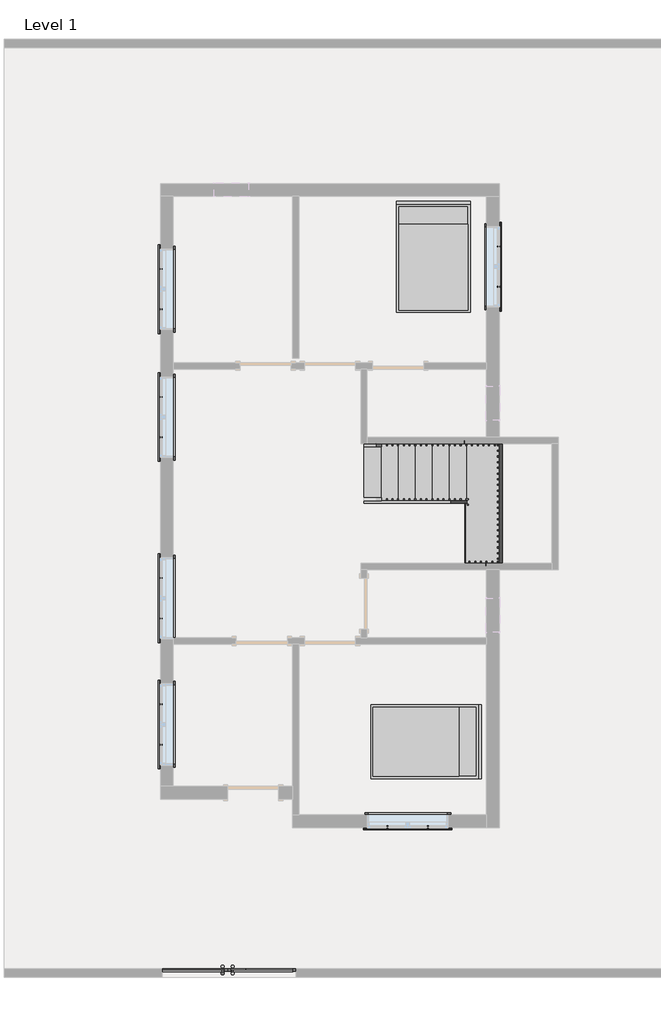
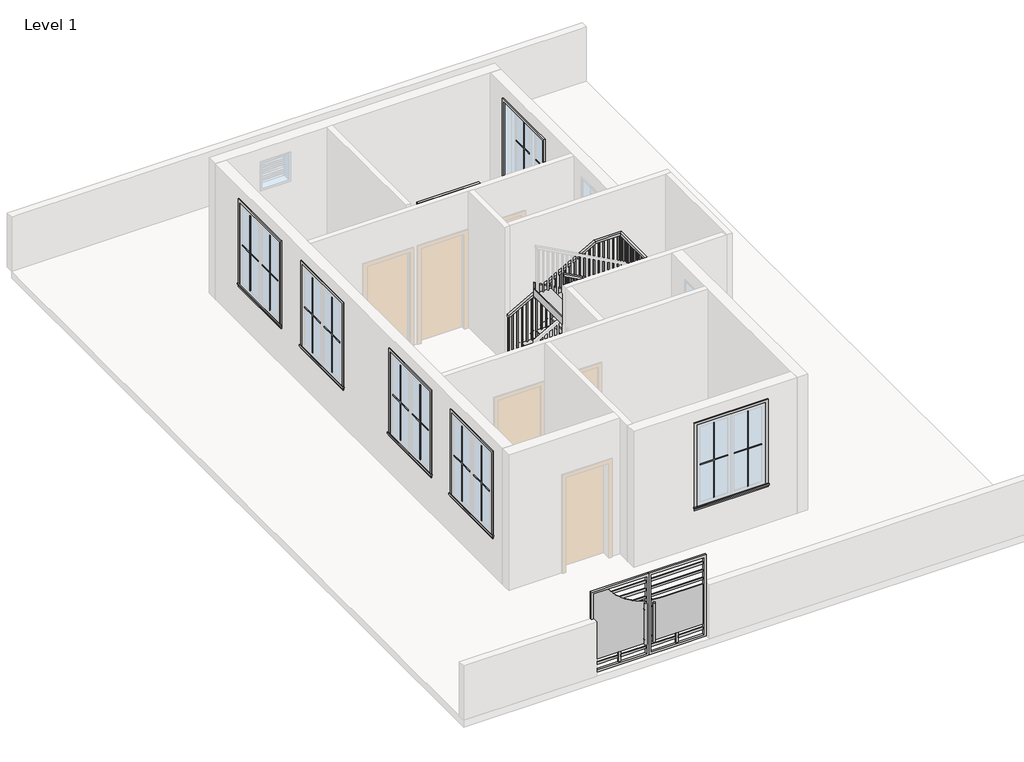
# One storey, part 2 of 2: 25 proxies, 5 members, 2 furniture elements, 1 railing, 1 stair flight.
"""IFC4 building model written with IfcOpenShell, lengths in millimetres."""

from ifc_helpers import new_model, si_unit, frame, origin, place, context, project, spatial, polyline, outline, extrude, faceted_brep, transform, mapped, element, save
from components import generic_models_113f6068, muntin_pattern_2x2_muntin_pattern_2x2_bff912c5, muntin_pattern_2x2_muntin_pattern_2x2_c2194282, trim_window_exterior_flat_with_sill_e04b3088, trim_window_interior_flat_picture_frame_2a7685fe, bed_17739_bed_17739_15c61121, stair_flight_5b4b54c9

model = new_model("IFC4")

# Units and contexts
model_context = context("Model", 3, world=origin())
ifc_project = project(units=[si_unit("LENGTHUNIT", "METRE", prefix="MILLI")], contexts=[model_context])

# Site, building, storey
site = spatial("IfcSite", under=ifc_project)
building = spatial("IfcBuilding", under=site)
storey = spatial("IfcBuildingStorey", under=building, Name="Level 1", Elevation=0.0)

# Proxies
placement = place(None, origin())
generic_models_shape = generic_models_113f6068(model_context)
element("IfcBuildingElementProxy", 1, Name="Generic Models", at=placement, inside=storey, context=model_context, shape_type="MappedRepresentation", body=[
    mapped(generic_models_shape, transform((-3606.0638307, -8534.8071204, 0.0), x_axis=(1.0, 0.0, 0.0), y_axis=(0.0, 1.0, 0.0), z_axis=(0.0, 0.0, 1.0))),
])
muntin_pattern_2x2_muntin_pattern_2x2_shape = muntin_pattern_2x2_muntin_pattern_2x2_bff912c5(model_context)
element("IfcBuildingElementProxy", 2, Name="Muntin Pattern_2x2 : Muntin Pattern_2x2", ObjectType="Muntin Pattern_2x2 : Muntin Pattern_2x2", at=placement, inside=storey, context=model_context, shape_type="MappedRepresentation", body=[
    mapped(muntin_pattern_2x2_muntin_pattern_2x2_shape, transform((-4796.6888307, -4528.6107799, 984.25), x_axis=(0.0, 1.0, 0.0), y_axis=(-1.0, 0.0, 0.0), z_axis=(0.0, 0.0, 1.0))),
])
element("IfcBuildingElementProxy", 3, Name="Muntin Pattern_2x2 : Muntin Pattern_2x2", ObjectType="Muntin Pattern_2x2 : Muntin Pattern_2x2", at=placement, inside=storey, context=model_context, shape_type="MappedRepresentation", body=[
    mapped(muntin_pattern_2x2_muntin_pattern_2x2_shape, transform((-4796.6888307, -2274.3607799, 984.25), x_axis=(0.0, 1.0, 0.0), y_axis=(-1.0, 0.0, 0.0), z_axis=(0.0, 0.0, 1.0))),
])
element("IfcBuildingElementProxy", 4, Name="Muntin Pattern_2x2 : Muntin Pattern_2x2", ObjectType="Muntin Pattern_2x2 : Muntin Pattern_2x2", at=placement, inside=storey, context=model_context, shape_type="MappedRepresentation", body=[
    mapped(muntin_pattern_2x2_muntin_pattern_2x2_shape, transform((-26.2513307, -6000.2232799, 984.25), x_axis=(-1.0, 0.0, 0.0), y_axis=(0.0, -1.0, 0.0), z_axis=(0.0, 0.0, 1.0))),
])
element("IfcBuildingElementProxy", 5, Name="Muntin Pattern_2x2 : Muntin Pattern_2x2", ObjectType="Muntin Pattern_2x2 : Muntin Pattern_2x2", at=placement, inside=storey, context=model_context, shape_type="MappedRepresentation", body=[
    mapped(muntin_pattern_2x2_muntin_pattern_2x2_shape, transform((1242.1611693, 4370.9142201, 984.25), x_axis=(0.0, -1.0, 0.0), y_axis=(1.0, 0.0, 0.0), z_axis=(0.0, 0.0, 1.0))),
])
element("IfcBuildingElementProxy", 6, Name="Muntin Pattern_2x2 : Muntin Pattern_2x2", ObjectType="Muntin Pattern_2x2 : Muntin Pattern_2x2", at=placement, inside=storey, context=model_context, shape_type="MappedRepresentation", body=[
    mapped(muntin_pattern_2x2_muntin_pattern_2x2_shape, transform((-4796.6888307, 3250.1392201, 984.25), x_axis=(0.0, 1.0, 0.0), y_axis=(-1.0, 0.0, 0.0), z_axis=(0.0, 0.0, 1.0))),
])
element("IfcBuildingElementProxy", 7, Name="Muntin Pattern_2x2 : Muntin Pattern_2x2", ObjectType="Muntin Pattern_2x2 : Muntin Pattern_2x2", at=placement, inside=storey, context=model_context, shape_type="MappedRepresentation", body=[
    mapped(muntin_pattern_2x2_muntin_pattern_2x2_shape, transform((-4796.6888307, 964.1392201, 984.25), x_axis=(0.0, 1.0, 0.0), y_axis=(-1.0, 0.0, 0.0), z_axis=(0.0, 0.0, 1.0))),
])
muntin_pattern_2x2_muntin_pattern_2x2_2_shape = muntin_pattern_2x2_muntin_pattern_2x2_c2194282(model_context)
element("IfcBuildingElementProxy", 8, Name="Muntin Pattern_2x2 : Muntin Pattern_2x2", ObjectType="Muntin Pattern_2x2 : Muntin Pattern_2x2", at=placement, inside=storey, context=model_context, shape_type="MappedRepresentation", body=[
    mapped(muntin_pattern_2x2_muntin_pattern_2x2_2_shape, transform((-4796.6888307, -3807.8857799, 984.25), x_axis=(0.0, -1.0, 0.0), y_axis=(1.0, 0.0, 0.0), z_axis=(0.0, 0.0, 1.0))),
])
element("IfcBuildingElementProxy", 9, Name="Muntin Pattern_2x2 : Muntin Pattern_2x2", ObjectType="Muntin Pattern_2x2 : Muntin Pattern_2x2", at=placement, inside=storey, context=model_context, shape_type="MappedRepresentation", body=[
    mapped(muntin_pattern_2x2_muntin_pattern_2x2_2_shape, transform((-4796.6888307, -1553.6357799, 984.25), x_axis=(0.0, -1.0, 0.0), y_axis=(1.0, 0.0, 0.0), z_axis=(0.0, 0.0, 1.0))),
])
element("IfcBuildingElementProxy", 10, Name="Muntin Pattern_2x2 : Muntin Pattern_2x2", ObjectType="Muntin Pattern_2x2 : Muntin Pattern_2x2", at=placement, inside=storey, context=model_context, shape_type="MappedRepresentation", body=[
    mapped(muntin_pattern_2x2_muntin_pattern_2x2_2_shape, transform((-746.9763307, -6000.2232799, 984.25), x_axis=(1.0, 0.0, 0.0), y_axis=(0.0, 1.0, 0.0), z_axis=(0.0, 0.0, 1.0))),
])
element("IfcBuildingElementProxy", 11, Name="Muntin Pattern_2x2 : Muntin Pattern_2x2", ObjectType="Muntin Pattern_2x2 : Muntin Pattern_2x2", at=placement, inside=storey, context=model_context, shape_type="MappedRepresentation", body=[
    mapped(muntin_pattern_2x2_muntin_pattern_2x2_2_shape, transform((1242.1611693, 3650.1892201, 984.25), x_axis=(0.0, 1.0, 0.0), y_axis=(-1.0, 0.0, 0.0), z_axis=(0.0, 0.0, 1.0))),
])
element("IfcBuildingElementProxy", 12, Name="Muntin Pattern_2x2 : Muntin Pattern_2x2", ObjectType="Muntin Pattern_2x2 : Muntin Pattern_2x2", at=placement, inside=storey, context=model_context, shape_type="MappedRepresentation", body=[
    mapped(muntin_pattern_2x2_muntin_pattern_2x2_2_shape, transform((-4796.6888307, 3970.8642201, 984.25), x_axis=(0.0, -1.0, 0.0), y_axis=(1.0, 0.0, 0.0), z_axis=(0.0, 0.0, 1.0))),
])
element("IfcBuildingElementProxy", 13, Name="Muntin Pattern_2x2 : Muntin Pattern_2x2", ObjectType="Muntin Pattern_2x2 : Muntin Pattern_2x2", at=placement, inside=storey, context=model_context, shape_type="MappedRepresentation", body=[
    mapped(muntin_pattern_2x2_muntin_pattern_2x2_2_shape, transform((-4796.6888307, 1684.8642201, 984.25), x_axis=(0.0, -1.0, 0.0), y_axis=(1.0, 0.0, 0.0), z_axis=(0.0, 0.0, 1.0))),
])
trim_window_exterior_flat_with_sill_shape = trim_window_exterior_flat_with_sill_e04b3088(model_context)
element("IfcBuildingElementProxy", 14, Name="Trim-Window-Exterior-Flat : with Sill", ObjectType="Trim-Window-Exterior-Flat : with Sill", at=placement, inside=storey, context=model_context, shape_type="MappedRepresentation", body=[
    mapped(trim_window_exterior_flat_with_sill_shape, transform((-4806.2138307, -4168.2482799, 2743.2), x_axis=(0.0, -1.0, 0.0), y_axis=(0.0, 0.0, 1.0), z_axis=(-1.0, 0.0, 0.0))),
])
element("IfcBuildingElementProxy", 15, Name="Trim-Window-Exterior-Flat : with Sill", ObjectType="Trim-Window-Exterior-Flat : with Sill", at=placement, inside=storey, context=model_context, shape_type="MappedRepresentation", body=[
    mapped(trim_window_exterior_flat_with_sill_shape, transform((-4806.2138307, -1913.9982799, 2743.2), x_axis=(0.0, -1.0, 0.0), y_axis=(0.0, 0.0, 1.0), z_axis=(-1.0, 0.0, 0.0))),
])
element("IfcBuildingElementProxy", 16, Name="Trim-Window-Exterior-Flat : with Sill", ObjectType="Trim-Window-Exterior-Flat : with Sill", at=placement, inside=storey, context=model_context, shape_type="MappedRepresentation", body=[
    mapped(trim_window_exterior_flat_with_sill_shape, transform((-386.6138307, -6009.7482799, 2743.2), x_axis=(1.0, 0.0, 0.0), y_axis=(0.0, 0.0, 1.0), z_axis=(0.0, -1.0, 0.0))),
])
element("IfcBuildingElementProxy", 17, Name="Trim-Window-Exterior-Flat : with Sill", ObjectType="Trim-Window-Exterior-Flat : with Sill", at=placement, inside=storey, context=model_context, shape_type="MappedRepresentation", body=[
    mapped(trim_window_exterior_flat_with_sill_shape, transform((1251.6861693, 4010.5517201, 2743.2), x_axis=(0.0, 1.0, 0.0), y_axis=(0.0, 0.0, 1.0), z_axis=(1.0, 0.0, 0.0))),
])
element("IfcBuildingElementProxy", 18, Name="Trim-Window-Exterior-Flat : with Sill", ObjectType="Trim-Window-Exterior-Flat : with Sill", at=placement, inside=storey, context=model_context, shape_type="MappedRepresentation", body=[
    mapped(trim_window_exterior_flat_with_sill_shape, transform((-4806.2138307, 3610.5017201, 2743.2), x_axis=(0.0, -1.0, 0.0), y_axis=(0.0, 0.0, 1.0), z_axis=(-1.0, 0.0, 0.0))),
])
element("IfcBuildingElementProxy", 19, Name="Trim-Window-Exterior-Flat : with Sill", ObjectType="Trim-Window-Exterior-Flat : with Sill", at=placement, inside=storey, context=model_context, shape_type="MappedRepresentation", body=[
    mapped(trim_window_exterior_flat_with_sill_shape, transform((-4806.2138307, 1324.5017201, 2743.2), x_axis=(0.0, -1.0, 0.0), y_axis=(0.0, 0.0, 1.0), z_axis=(-1.0, 0.0, 0.0))),
])
trim_window_interior_flat_picture_frame_shape = trim_window_interior_flat_picture_frame_2a7685fe(model_context)
element("IfcBuildingElementProxy", 20, Name="Trim-Window-Interior-Flat : Picture Frame", ObjectType="Trim-Window-Interior-Flat : Picture Frame", at=placement, inside=storey, context=model_context, shape_type="MappedRepresentation", body=[
    mapped(trim_window_interior_flat_picture_frame_shape, transform((-4577.6138307, -4168.2482799, 2743.2), x_axis=(0.0, 1.0, 0.0), y_axis=(0.0, 0.0, 1.0), z_axis=(1.0, 0.0, 0.0))),
])
element("IfcBuildingElementProxy", 21, Name="Trim-Window-Interior-Flat : Picture Frame", ObjectType="Trim-Window-Interior-Flat : Picture Frame", at=placement, inside=storey, context=model_context, shape_type="MappedRepresentation", body=[
    mapped(trim_window_interior_flat_picture_frame_shape, transform((-4577.6138307, -1913.9982799, 2743.2), x_axis=(0.0, 1.0, 0.0), y_axis=(0.0, 0.0, 1.0), z_axis=(1.0, 0.0, 0.0))),
])
element("IfcBuildingElementProxy", 22, Name="Trim-Window-Interior-Flat : Picture Frame", ObjectType="Trim-Window-Interior-Flat : Picture Frame", at=placement, inside=storey, context=model_context, shape_type="MappedRepresentation", body=[
    mapped(trim_window_interior_flat_picture_frame_shape, transform((-386.6138307, -5781.1482799, 2743.2), x_axis=(-1.0, 0.0, 0.0), y_axis=(0.0, 0.0, 1.0), z_axis=(0.0, 1.0, 0.0))),
])
element("IfcBuildingElementProxy", 23, Name="Trim-Window-Interior-Flat : Picture Frame", ObjectType="Trim-Window-Interior-Flat : Picture Frame", at=placement, inside=storey, context=model_context, shape_type="MappedRepresentation", body=[
    mapped(trim_window_interior_flat_picture_frame_shape, transform((1023.0861693, 4010.5517201, 2743.2), x_axis=(0.0, -1.0, 0.0), y_axis=(0.0, 0.0, 1.0), z_axis=(-1.0, 0.0, 0.0))),
])
element("IfcBuildingElementProxy", 24, Name="Trim-Window-Interior-Flat : Picture Frame", ObjectType="Trim-Window-Interior-Flat : Picture Frame", at=placement, inside=storey, context=model_context, shape_type="MappedRepresentation", body=[
    mapped(trim_window_interior_flat_picture_frame_shape, transform((-4577.6138307, 3610.5017201, 2743.2), x_axis=(0.0, 1.0, 0.0), y_axis=(0.0, 0.0, 1.0), z_axis=(1.0, 0.0, 0.0))),
])
element("IfcBuildingElementProxy", 25, Name="Trim-Window-Interior-Flat : Picture Frame", ObjectType="Trim-Window-Interior-Flat : Picture Frame", at=placement, inside=storey, context=model_context, shape_type="MappedRepresentation", body=[
    mapped(trim_window_interior_flat_picture_frame_shape, transform((-4577.6138307, 1324.5017201, 2743.2), x_axis=(0.0, 1.0, 0.0), y_axis=(0.0, 0.0, 1.0), z_axis=(1.0, 0.0, 0.0))),
])

# Furniture
bed_17739_bed_17739_shape = bed_17739_bed_17739_15c61121(model_context)
element("IfcFurniture", 26, ObjectType="Bed_17739 : Bed_17739", at=placement, inside=storey, context=model_context, shape_type="MappedRepresentation", body=[
    mapped(bed_17739_bed_17739_shape, transform((70.5861693, 4162.9517201, 0.0), x_axis=(1.0, 0.0, 0.0), y_axis=(0.0, 1.0, 0.0), z_axis=(0.0, 0.0, 1.0))),
])
element("IfcFurniture", 27, ObjectType="Bed_17739 : Bed_17739", at=placement, inside=storey, context=model_context, shape_type="MappedRepresentation", body=[
    mapped(bed_17739_bed_17739_shape, transform((-81.8138307, -4473.0482799, 0.0), x_axis=(0.0, -1.0, 0.0), y_axis=(1.0, 0.0, 0.0), z_axis=(0.0, 0.0, 1.0))),
])

# Members
element("IfcMember", 28, ObjectType="Stringer - 2\" Width", at=placement, inside=storey, context=model_context, shape_type="SweptSolid", body=[
    extrude(outline(polyline([(204.070617, -1167.6638307), (0.0, -1167.6638307), (0.0, -907.3693279), (1199.4752762, 1251.6861693), (1261.5333333, 1251.6861693), (1261.5333333, 735.7690587), (204.070617, -1167.6638307)])), frame((0.0, 848.2517201, 0.0), z_axis=(0.0, 1.0, 0.0), x_axis=(0.0, 0.0, 1.0)), (0.0, 0.0, 1.0), 50.8),
])
element("IfcMember", 29, ObjectType="Stringer - 2\" Width", at=placement, inside=storey, context=model_context, shape_type="SweptSolid", body=[
    extrude(outline(polyline([(1251.6861693, 899.0517201), (1302.4861693, 899.0517201), (1302.4861693, -1285.3482799), (1251.6861693, -1285.3482799), (1251.6861693, 899.0517201)])), frame((0.0, 0.0, 956.7333333), z_axis=(0.0, 0.0, 1.0), x_axis=(1.0, 0.0, 0.0)), (0.0, 0.0, 1.0), 304.8),
])
element("IfcMember", 30, ObjectType="Stringer - 2\" Width", at=placement, inside=storey, context=model_context, shape_type="SweptSolid", body=[
    extrude(outline(polyline([(956.7333333, 1302.4861693), (1040.1539503, 1302.4861693), (2423.0428392, -1186.7138307), (2074.3641651, -1186.7138307), (956.7333333, 825.0216665), (956.7333333, 1302.4861693)])), frame((0.0, -1336.1482799, 0.0), z_axis=(0.0, 1.0, 0.0), x_axis=(0.0, 0.0, 1.0)), (0.0, 0.0, 1.0), 50.8),
])
element("IfcMember", 31, ObjectType="Stringer - 2\" Width", at=placement, inside=storey, context=model_context, shape_type="SweptSolid", body=[
    extrude(outline(polyline([(204.070617, -1167.6638307), (0.0, -1167.6638307), (0.0, -907.3693279), (846.6974984, 616.6861693), (1195.3761726, 616.6861693), (204.070617, -1167.6638307)])), frame((0.0, -218.5482799, 0.0), z_axis=(0.0, 1.0, 0.0), x_axis=(0.0, 0.0, 1.0)), (0.0, 0.0, 1.0), 50.8),
])
element("IfcMember", 32, ObjectType="Stringer - 2\" Width", at=placement, inside=storey, context=model_context, shape_type="SweptSolid", body=[
    extrude(outline(polyline([(1044.253054, 667.4861693), (1392.9317281, 667.4861693), (2423.0428392, -1186.7138307), (2074.3641651, -1186.7138307), (1044.253054, 667.4861693)])), frame((0.0, -218.5482799, 0.0), z_axis=(0.0, 1.0, 0.0), x_axis=(0.0, 0.0, 1.0)), (0.0, 0.0, 1.0), 50.8),
])

# Railing
element("IfcRailing", 33, ObjectType="Handrail - Rectangular", at=placement, inside=storey, context=model_context, shape_type="SolidModel", body=[
    faceted_brep([(-1167.6638307, 848.2517201, 1083.7333333), (-1167.6638307, 848.2517201, 1025.6675836), (-1167.6638307, 797.4517201, 1025.6675836), (-1167.6638307, 797.4517201, 1083.7333333), (667.4861693, 848.2517201, 2099.7333333), (680.6099298, 848.2517201, 2048.9333333), (680.6099298, 797.4517201, 2048.9333333), (667.4861693, 797.4517201, 2099.7333333), (1251.6861693, 848.2517201, 2099.7333333), (1251.6861693, 848.2517201, 2048.9333333), (1200.8861693, 797.4517201, 2048.9333333), (1200.8861693, 797.4517201, 2099.7333333), (1251.6861693, -1285.3482799, 2099.7333333), (1251.6861693, -1285.3482799, 2048.9333333), (1200.8861693, -1234.5482799, 2048.9333333), (1200.8861693, -1234.5482799, 2099.7333333), (976.5195026, -1285.3482799, 2099.7333333), (963.5139215, -1285.3482799, 2048.9333333), (963.5139215, -1234.5482799, 2048.9333333), (976.5195026, -1234.5482799, 2099.7333333), (-1186.7138307, -1285.3482799, 3285.0666667), (-1186.7138307, -1234.5482799, 3285.0666667), (-1186.7138307, -1234.5482799, 3227.1403208), (-1186.7138307, -1285.3482799, 3227.1403208)], [[[0, 1, 2, 3]], [[1, 0, 4, 5]], [[2, 1, 5, 6]], [[3, 2, 6, 7]], [[0, 3, 7, 4]], [[5, 4, 8, 9]], [[6, 5, 9, 10]], [[7, 6, 10, 11]], [[4, 7, 11, 8]], [[9, 8, 12, 13]], [[10, 9, 13, 14]], [[11, 10, 14, 15]], [[8, 11, 15, 12]], [[13, 12, 16, 17]], [[14, 13, 17, 18]], [[15, 14, 18, 19]], [[12, 15, 19, 16]], [[20, 21, 22, 23]], [[17, 16, 20, 23]], [[18, 17, 23, 22]], [[19, 18, 22, 21]], [[16, 19, 21, 20]]]),
    extrude(outline(polyline([(3190.6060742, -1120.0388307), (2201.3333333, -1120.0388307), (2201.3333333, -1100.9888307), (3180.1677181, -1100.9888307), (3190.6060742, -1120.0388307)])), frame((0.0, -1269.4732799, 0.0), z_axis=(0.0, 1.0, 0.0), x_axis=(0.0, 0.0, 1.0)), (0.0, 0.0, 1.0), 19.05),
    extrude(outline(polyline([(3134.9348414, -1018.4388307), (2201.3333333, -1018.4388307), (2201.3333333, -999.3888307), (3124.4964852, -999.3888307), (3134.9348414, -1018.4388307)])), frame((0.0, -1269.4732799, 0.0), z_axis=(0.0, 1.0, 0.0), x_axis=(0.0, 0.0, 1.0)), (0.0, 0.0, 1.0), 19.05),
    extrude(outline(polyline([(3079.2636085, -916.8388307), (2201.3333333, -916.8388307), (2201.3333333, -897.7888307), (3068.8252523, -897.7888307), (3079.2636085, -916.8388307)])), frame((0.0, -1269.4732799, 0.0), z_axis=(0.0, 1.0, 0.0), x_axis=(0.0, 0.0, 1.0)), (0.0, 0.0, 1.0), 19.05),
    extrude(outline(polyline([(3023.5923756, -815.2388307), (2032.0, -815.2388307), (2032.0, -796.1888307), (3013.1540195, -796.1888307), (3023.5923756, -815.2388307)])), frame((0.0, -1269.4732799, 0.0), z_axis=(0.0, 1.0, 0.0), x_axis=(0.0, 0.0, 1.0)), (0.0, 0.0, 1.0), 19.05),
    extrude(outline(polyline([(2967.9211427, -713.6388307), (2032.0, -713.6388307), (2032.0, -694.5888307), (2957.4827866, -694.5888307), (2967.9211427, -713.6388307)])), frame((0.0, -1269.4732799, 0.0), z_axis=(0.0, 1.0, 0.0), x_axis=(0.0, 0.0, 1.0)), (0.0, 0.0, 1.0), 19.05),
    extrude(outline(polyline([(2912.2499099, -612.0388307), (2032.0, -612.0388307), (2032.0, -592.9888307), (2901.8115537, -592.9888307), (2912.2499099, -612.0388307)])), frame((0.0, -1269.4732799, 0.0), z_axis=(0.0, 1.0, 0.0), x_axis=(0.0, 0.0, 1.0)), (0.0, 0.0, 1.0), 19.05),
    extrude(outline(polyline([(2856.578677, -510.4388307), (1862.6666667, -510.4388307), (1862.6666667, -491.3888307), (2846.1403208, -491.3888307), (2856.578677, -510.4388307)])), frame((0.0, -1269.4732799, 0.0), z_axis=(0.0, 1.0, 0.0), x_axis=(0.0, 0.0, 1.0)), (0.0, 0.0, 1.0), 19.05),
    extrude(outline(polyline([(2800.9074441, -408.8388307), (1862.6666667, -408.8388307), (1862.6666667, -389.7888307), (2790.4690879, -389.7888307), (2800.9074441, -408.8388307)])), frame((0.0, -1269.4732799, 0.0), z_axis=(0.0, 1.0, 0.0), x_axis=(0.0, 0.0, 1.0)), (0.0, 0.0, 1.0), 19.05),
    extrude(outline(polyline([(2745.2362112, -307.2388307), (1862.6666667, -307.2388307), (1862.6666667, -288.1888307), (2734.7978551, -288.1888307), (2745.2362112, -307.2388307)])), frame((0.0, -1269.4732799, 0.0), z_axis=(0.0, 1.0, 0.0), x_axis=(0.0, 0.0, 1.0)), (0.0, 0.0, 1.0), 19.05),
    extrude(outline(polyline([(2689.5649784, -205.6388307), (1693.3333333, -205.6388307), (1693.3333333, -186.5888307), (2679.1266222, -186.5888307), (2689.5649784, -205.6388307)])), frame((0.0, -1269.4732799, 0.0), z_axis=(0.0, 1.0, 0.0), x_axis=(0.0, 0.0, 1.0)), (0.0, 0.0, 1.0), 19.05),
    extrude(outline(polyline([(2633.8937455, -104.0388307), (1693.3333333, -104.0388307), (1693.3333333, -84.9888307), (2623.4553893, -84.9888307), (2633.8937455, -104.0388307)])), frame((0.0, -1269.4732799, 0.0), z_axis=(0.0, 1.0, 0.0), x_axis=(0.0, 0.0, 1.0)), (0.0, 0.0, 1.0), 19.05),
    extrude(outline(polyline([(2578.2225126, -2.4388307), (1693.3333333, -2.4388307), (1693.3333333, 16.6111693), (2567.7841564, 16.6111693), (2578.2225126, -2.4388307)])), frame((0.0, -1269.4732799, 0.0), z_axis=(0.0, 1.0, 0.0), x_axis=(0.0, 0.0, 1.0)), (0.0, 0.0, 1.0), 19.05),
    extrude(outline(polyline([(2522.5512797, 99.1611693), (1524.0, 99.1611693), (1524.0, 118.2111693), (2512.1129236, 118.2111693), (2522.5512797, 99.1611693)])), frame((0.0, -1269.4732799, 0.0), z_axis=(0.0, 1.0, 0.0), x_axis=(0.0, 0.0, 1.0)), (0.0, 0.0, 1.0), 19.05),
    extrude(outline(polyline([(2466.8800469, 200.7611693), (1524.0, 200.7611693), (1524.0, 219.8111693), (2456.4416907, 219.8111693), (2466.8800469, 200.7611693)])), frame((0.0, -1269.4732799, 0.0), z_axis=(0.0, 1.0, 0.0), x_axis=(0.0, 0.0, 1.0)), (0.0, 0.0, 1.0), 19.05),
    extrude(outline(polyline([(2411.208814, 302.3611693), (1524.0, 302.3611693), (1524.0, 321.4111693), (2400.7704578, 321.4111693), (2411.208814, 302.3611693)])), frame((0.0, -1269.4732799, 0.0), z_axis=(0.0, 1.0, 0.0), x_axis=(0.0, 0.0, 1.0)), (0.0, 0.0, 1.0), 19.05),
    extrude(outline(polyline([(2355.5375811, 403.9611693), (1354.6666667, 403.9611693), (1354.6666667, 423.0111693), (2345.0992249, 423.0111693), (2355.5375811, 403.9611693)])), frame((0.0, -1269.4732799, 0.0), z_axis=(0.0, 1.0, 0.0), x_axis=(0.0, 0.0, 1.0)), (0.0, 0.0, 1.0), 19.05),
    extrude(outline(polyline([(2299.8663482, 505.5611693), (1354.6666667, 505.5611693), (1354.6666667, 524.6111693), (2289.4279921, 524.6111693), (2299.8663482, 505.5611693)])), frame((0.0, -1269.4732799, 0.0), z_axis=(0.0, 1.0, 0.0), x_axis=(0.0, 0.0, 1.0)), (0.0, 0.0, 1.0), 19.05),
    extrude(outline(polyline([(2244.1951153, 607.1611693), (1354.6666667, 607.1611693), (1354.6666667, 626.2111693), (2233.7567592, 626.2111693), (2244.1951153, 607.1611693)])), frame((0.0, -1269.4732799, 0.0), z_axis=(0.0, 1.0, 0.0), x_axis=(0.0, 0.0, 1.0)), (0.0, 0.0, 1.0), 19.05),
    extrude(outline(polyline([(2188.5238825, 708.7611693), (1185.3333333, 708.7611693), (1185.3333333, 727.8111693), (2178.0855263, 727.8111693), (2188.5238825, 708.7611693)])), frame((0.0, -1269.4732799, 0.0), z_axis=(0.0, 1.0, 0.0), x_axis=(0.0, 0.0, 1.0)), (0.0, 0.0, 1.0), 19.05),
    extrude(outline(polyline([(2132.8526496, 810.3611693), (1185.3333333, 810.3611693), (1185.3333333, 829.4111693), (2122.4142934, 829.4111693), (2132.8526496, 810.3611693)])), frame((0.0, -1269.4732799, 0.0), z_axis=(0.0, 1.0, 0.0), x_axis=(0.0, 0.0, 1.0)), (0.0, 0.0, 1.0), 19.05),
    extrude(outline(polyline([(2077.1814167, 911.9611693), (1185.3333333, 911.9611693), (1185.3333333, 931.0111693), (2066.7430606, 931.0111693), (2077.1814167, 911.9611693)])), frame((0.0, -1269.4732799, 0.0), z_axis=(0.0, 1.0, 0.0), x_axis=(0.0, 0.0, 1.0)), (0.0, 0.0, 1.0), 19.05),
    extrude(outline(polyline([(1032.6111693, -1269.4732799), (1013.5611693, -1269.4732799), (1013.5611693, -1250.4232799), (1032.6111693, -1250.4232799), (1032.6111693, -1269.4732799)])), frame((0.0, 0.0, 1185.3333333), z_axis=(0.0, 0.0, 1.0), x_axis=(1.0, 0.0, 0.0)), (0.0, 0.0, 1.0), 863.6),
    extrude(outline(polyline([(1134.2111693, -1269.4732799), (1115.1611693, -1269.4732799), (1115.1611693, -1250.4232799), (1134.2111693, -1250.4232799), (1134.2111693, -1269.4732799)])), frame((0.0, 0.0, 1185.3333333), z_axis=(0.0, 0.0, 1.0), x_axis=(1.0, 0.0, 0.0)), (0.0, 0.0, 1.0), 863.6),
    extrude(outline(polyline([(1235.8111693, -1199.6232799), (1235.8111693, -1218.6732799), (1216.7611693, -1218.6732799), (1216.7611693, -1199.6232799), (1235.8111693, -1199.6232799)])), frame((0.0, 0.0, 1185.3333333), z_axis=(0.0, 0.0, 1.0), x_axis=(1.0, 0.0, 0.0)), (0.0, 0.0, 1.0), 863.6),
    extrude(outline(polyline([(1235.8111693, -1098.0232799), (1235.8111693, -1117.0732799), (1216.7611693, -1117.0732799), (1216.7611693, -1098.0232799), (1235.8111693, -1098.0232799)])), frame((0.0, 0.0, 1185.3333333), z_axis=(0.0, 0.0, 1.0), x_axis=(1.0, 0.0, 0.0)), (0.0, 0.0, 1.0), 863.6),
    extrude(outline(polyline([(1235.8111693, -996.4232799), (1235.8111693, -1015.4732799), (1216.7611693, -1015.4732799), (1216.7611693, -996.4232799), (1235.8111693, -996.4232799)])), frame((0.0, 0.0, 1185.3333333), z_axis=(0.0, 0.0, 1.0), x_axis=(1.0, 0.0, 0.0)), (0.0, 0.0, 1.0), 863.6),
    extrude(outline(polyline([(1235.8111693, -894.8232799), (1235.8111693, -913.8732799), (1216.7611693, -913.8732799), (1216.7611693, -894.8232799), (1235.8111693, -894.8232799)])), frame((0.0, 0.0, 1185.3333333), z_axis=(0.0, 0.0, 1.0), x_axis=(1.0, 0.0, 0.0)), (0.0, 0.0, 1.0), 863.6),
    extrude(outline(polyline([(1235.8111693, -793.2232799), (1235.8111693, -812.2732799), (1216.7611693, -812.2732799), (1216.7611693, -793.2232799), (1235.8111693, -793.2232799)])), frame((0.0, 0.0, 1185.3333333), z_axis=(0.0, 0.0, 1.0), x_axis=(1.0, 0.0, 0.0)), (0.0, 0.0, 1.0), 863.6),
    extrude(outline(polyline([(1235.8111693, -691.6232799), (1235.8111693, -710.6732799), (1216.7611693, -710.6732799), (1216.7611693, -691.6232799), (1235.8111693, -691.6232799)])), frame((0.0, 0.0, 1185.3333333), z_axis=(0.0, 0.0, 1.0), x_axis=(1.0, 0.0, 0.0)), (0.0, 0.0, 1.0), 863.6),
    extrude(outline(polyline([(1235.8111693, -590.0232799), (1235.8111693, -609.0732799), (1216.7611693, -609.0732799), (1216.7611693, -590.0232799), (1235.8111693, -590.0232799)])), frame((0.0, 0.0, 1185.3333333), z_axis=(0.0, 0.0, 1.0), x_axis=(1.0, 0.0, 0.0)), (0.0, 0.0, 1.0), 863.6),
    extrude(outline(polyline([(1235.8111693, -488.4232799), (1235.8111693, -507.4732799), (1216.7611693, -507.4732799), (1216.7611693, -488.4232799), (1235.8111693, -488.4232799)])), frame((0.0, 0.0, 1185.3333333), z_axis=(0.0, 0.0, 1.0), x_axis=(1.0, 0.0, 0.0)), (0.0, 0.0, 1.0), 863.6),
    extrude(outline(polyline([(1235.8111693, -386.8232799), (1235.8111693, -405.8732799), (1216.7611693, -405.8732799), (1216.7611693, -386.8232799), (1235.8111693, -386.8232799)])), frame((0.0, 0.0, 1185.3333333), z_axis=(0.0, 0.0, 1.0), x_axis=(1.0, 0.0, 0.0)), (0.0, 0.0, 1.0), 863.6),
    extrude(outline(polyline([(1235.8111693, -285.2232799), (1235.8111693, -304.2732799), (1216.7611693, -304.2732799), (1216.7611693, -285.2232799), (1235.8111693, -285.2232799)])), frame((0.0, 0.0, 1185.3333333), z_axis=(0.0, 0.0, 1.0), x_axis=(1.0, 0.0, 0.0)), (0.0, 0.0, 1.0), 863.6),
    extrude(outline(polyline([(1235.8111693, -183.6232799), (1235.8111693, -202.6732799), (1216.7611693, -202.6732799), (1216.7611693, -183.6232799), (1235.8111693, -183.6232799)])), frame((0.0, 0.0, 1185.3333333), z_axis=(0.0, 0.0, 1.0), x_axis=(1.0, 0.0, 0.0)), (0.0, 0.0, 1.0), 863.6),
    extrude(outline(polyline([(1235.8111693, -82.0232799), (1235.8111693, -101.0732799), (1216.7611693, -101.0732799), (1216.7611693, -82.0232799), (1235.8111693, -82.0232799)])), frame((0.0, 0.0, 1185.3333333), z_axis=(0.0, 0.0, 1.0), x_axis=(1.0, 0.0, 0.0)), (0.0, 0.0, 1.0), 863.6),
    extrude(outline(polyline([(1235.8111693, 19.5767201), (1235.8111693, 0.5267201), (1216.7611693, 0.5267201), (1216.7611693, 19.5767201), (1235.8111693, 19.5767201)])), frame((0.0, 0.0, 1185.3333333), z_axis=(0.0, 0.0, 1.0), x_axis=(1.0, 0.0, 0.0)), (0.0, 0.0, 1.0), 863.6),
    extrude(outline(polyline([(1235.8111693, 121.1767201), (1235.8111693, 102.1267201), (1216.7611693, 102.1267201), (1216.7611693, 121.1767201), (1235.8111693, 121.1767201)])), frame((0.0, 0.0, 1185.3333333), z_axis=(0.0, 0.0, 1.0), x_axis=(1.0, 0.0, 0.0)), (0.0, 0.0, 1.0), 863.6),
    extrude(outline(polyline([(1235.8111693, 222.7767201), (1235.8111693, 203.7267201), (1216.7611693, 203.7267201), (1216.7611693, 222.7767201), (1235.8111693, 222.7767201)])), frame((0.0, 0.0, 1185.3333333), z_axis=(0.0, 0.0, 1.0), x_axis=(1.0, 0.0, 0.0)), (0.0, 0.0, 1.0), 863.6),
    extrude(outline(polyline([(1235.8111693, 324.3767201), (1235.8111693, 305.3267201), (1216.7611693, 305.3267201), (1216.7611693, 324.3767201), (1235.8111693, 324.3767201)])), frame((0.0, 0.0, 1185.3333333), z_axis=(0.0, 0.0, 1.0), x_axis=(1.0, 0.0, 0.0)), (0.0, 0.0, 1.0), 863.6),
    extrude(outline(polyline([(1235.8111693, 425.9767201), (1235.8111693, 406.9267201), (1216.7611693, 406.9267201), (1216.7611693, 425.9767201), (1235.8111693, 425.9767201)])), frame((0.0, 0.0, 1185.3333333), z_axis=(0.0, 0.0, 1.0), x_axis=(1.0, 0.0, 0.0)), (0.0, 0.0, 1.0), 863.6),
    extrude(outline(polyline([(1235.8111693, 527.5767201), (1235.8111693, 508.5267201), (1216.7611693, 508.5267201), (1216.7611693, 527.5767201), (1235.8111693, 527.5767201)])), frame((0.0, 0.0, 1185.3333333), z_axis=(0.0, 0.0, 1.0), x_axis=(1.0, 0.0, 0.0)), (0.0, 0.0, 1.0), 863.6),
    extrude(outline(polyline([(1235.8111693, 629.1767201), (1235.8111693, 610.1267201), (1216.7611693, 610.1267201), (1216.7611693, 629.1767201), (1235.8111693, 629.1767201)])), frame((0.0, 0.0, 1185.3333333), z_axis=(0.0, 0.0, 1.0), x_axis=(1.0, 0.0, 0.0)), (0.0, 0.0, 1.0), 863.6),
    extrude(outline(polyline([(1235.8111693, 730.7767201), (1235.8111693, 711.7267201), (1216.7611693, 711.7267201), (1216.7611693, 730.7767201), (1235.8111693, 730.7767201)])), frame((0.0, 0.0, 1185.3333333), z_axis=(0.0, 0.0, 1.0), x_axis=(1.0, 0.0, 0.0)), (0.0, 0.0, 1.0), 863.6),
    extrude(outline(polyline([(1159.6111693, 832.3767201), (1178.6611693, 832.3767201), (1178.6611693, 813.3267201), (1159.6111693, 813.3267201), (1159.6111693, 832.3767201)])), frame((0.0, 0.0, 1185.3333333), z_axis=(0.0, 0.0, 1.0), x_axis=(1.0, 0.0, 0.0)), (0.0, 0.0, 1.0), 863.6),
    extrude(outline(polyline([(1058.0111693, 832.3767201), (1077.0611693, 832.3767201), (1077.0611693, 813.3267201), (1058.0111693, 813.3267201), (1058.0111693, 832.3767201)])), frame((0.0, 0.0, 1185.3333333), z_axis=(0.0, 0.0, 1.0), x_axis=(1.0, 0.0, 0.0)), (0.0, 0.0, 1.0), 863.6),
    extrude(outline(polyline([(956.4111693, 832.3767201), (975.4611693, 832.3767201), (975.4611693, 813.3267201), (956.4111693, 813.3267201), (956.4111693, 832.3767201)])), frame((0.0, 0.0, 1185.3333333), z_axis=(0.0, 0.0, 1.0), x_axis=(1.0, 0.0, 0.0)), (0.0, 0.0, 1.0), 863.6),
    extrude(outline(polyline([(854.8111693, 832.3767201), (873.8611693, 832.3767201), (873.8611693, 813.3267201), (854.8111693, 813.3267201), (854.8111693, 832.3767201)])), frame((0.0, 0.0, 1185.3333333), z_axis=(0.0, 0.0, 1.0), x_axis=(1.0, 0.0, 0.0)), (0.0, 0.0, 1.0), 863.6),
    extrude(outline(polyline([(753.2111693, 832.3767201), (772.2611693, 832.3767201), (772.2611693, 813.3267201), (753.2111693, 813.3267201), (753.2111693, 832.3767201)])), frame((0.0, 0.0, 1185.3333333), z_axis=(0.0, 0.0, 1.0), x_axis=(1.0, 0.0, 0.0)), (0.0, 0.0, 1.0), 863.6),
    extrude(outline(polyline([(2032.8786562, 651.6111693), (1016.0, 651.6111693), (1016.0, 670.6611693), (2043.425369, 670.6611693), (2032.8786562, 651.6111693)])), frame((0.0, 813.3267201, 0.0), z_axis=(0.0, 1.0, 0.0), x_axis=(0.0, 0.0, 1.0)), (0.0, 0.0, 1.0), 19.05),
    extrude(outline(polyline([(1976.6295213, 550.0111693), (1016.0, 550.0111693), (1016.0, 569.0611693), (1987.1762341, 569.0611693), (1976.6295213, 550.0111693)])), frame((0.0, 813.3267201, 0.0), z_axis=(0.0, 1.0, 0.0), x_axis=(0.0, 0.0, 1.0)), (0.0, 0.0, 1.0), 19.05),
    extrude(outline(polyline([(1920.3803863, 448.4111693), (1016.0, 448.4111693), (1016.0, 467.4611693), (1930.9270991, 467.4611693), (1920.3803863, 448.4111693)])), frame((0.0, 813.3267201, 0.0), z_axis=(0.0, 1.0, 0.0), x_axis=(0.0, 0.0, 1.0)), (0.0, 0.0, 1.0), 19.05),
    extrude(outline(polyline([(1864.1312514, 346.8111693), (846.6666667, 346.8111693), (846.6666667, 365.8611693), (1874.6779642, 365.8611693), (1864.1312514, 346.8111693)])), frame((0.0, 813.3267201, 0.0), z_axis=(0.0, 1.0, 0.0), x_axis=(0.0, 0.0, 1.0)), (0.0, 0.0, 1.0), 19.05),
    extrude(outline(polyline([(1807.8821164, 245.2111693), (846.6666667, 245.2111693), (846.6666667, 264.2611693), (1818.4288292, 264.2611693), (1807.8821164, 245.2111693)])), frame((0.0, 813.3267201, 0.0), z_axis=(0.0, 1.0, 0.0), x_axis=(0.0, 0.0, 1.0)), (0.0, 0.0, 1.0), 19.05),
    extrude(outline(polyline([(1751.6329815, 143.6111693), (846.6666667, 143.6111693), (846.6666667, 162.6611693), (1762.1796943, 162.6611693), (1751.6329815, 143.6111693)])), frame((0.0, 813.3267201, 0.0), z_axis=(0.0, 1.0, 0.0), x_axis=(0.0, 0.0, 1.0)), (0.0, 0.0, 1.0), 19.05),
    extrude(outline(polyline([(1695.3838465, 42.0111693), (677.3333333, 42.0111693), (677.3333333, 61.0611693), (1705.9305593, 61.0611693), (1695.3838465, 42.0111693)])), frame((0.0, 813.3267201, 0.0), z_axis=(0.0, 1.0, 0.0), x_axis=(0.0, 0.0, 1.0)), (0.0, 0.0, 1.0), 19.05),
    extrude(outline(polyline([(1639.1347116, -59.5888307), (677.3333333, -59.5888307), (677.3333333, -40.5388307), (1649.6814244, -40.5388307), (1639.1347116, -59.5888307)])), frame((0.0, 813.3267201, 0.0), z_axis=(0.0, 1.0, 0.0), x_axis=(0.0, 0.0, 1.0)), (0.0, 0.0, 1.0), 19.05),
    extrude(outline(polyline([(1582.8855766, -161.1888307), (677.3333333, -161.1888307), (677.3333333, -142.1388307), (1593.4322895, -142.1388307), (1582.8855766, -161.1888307)])), frame((0.0, 813.3267201, 0.0), z_axis=(0.0, 1.0, 0.0), x_axis=(0.0, 0.0, 1.0)), (0.0, 0.0, 1.0), 19.05),
    extrude(outline(polyline([(1526.6364417, -262.7888307), (508.0, -262.7888307), (508.0, -243.7388307), (1537.1831545, -243.7388307), (1526.6364417, -262.7888307)])), frame((0.0, 813.3267201, 0.0), z_axis=(0.0, 1.0, 0.0), x_axis=(0.0, 0.0, 1.0)), (0.0, 0.0, 1.0), 19.05),
    extrude(outline(polyline([(1470.3873068, -364.3888307), (508.0, -364.3888307), (508.0, -345.3388307), (1480.9340196, -345.3388307), (1470.3873068, -364.3888307)])), frame((0.0, 813.3267201, 0.0), z_axis=(0.0, 1.0, 0.0), x_axis=(0.0, 0.0, 1.0)), (0.0, 0.0, 1.0), 19.05),
    extrude(outline(polyline([(1414.1381718, -465.9888307), (508.0, -465.9888307), (508.0, -446.9388307), (1424.6848846, -446.9388307), (1414.1381718, -465.9888307)])), frame((0.0, 813.3267201, 0.0), z_axis=(0.0, 1.0, 0.0), x_axis=(0.0, 0.0, 1.0)), (0.0, 0.0, 1.0), 19.05),
    extrude(outline(polyline([(1357.8890369, -567.5888307), (338.6666667, -567.5888307), (338.6666667, -548.5388307), (1368.4357497, -548.5388307), (1357.8890369, -567.5888307)])), frame((0.0, 813.3267201, 0.0), z_axis=(0.0, 1.0, 0.0), x_axis=(0.0, 0.0, 1.0)), (0.0, 0.0, 1.0), 19.05),
    extrude(outline(polyline([(1301.6399019, -669.1888307), (338.6666667, -669.1888307), (338.6666667, -650.1388307), (1312.1866147, -650.1388307), (1301.6399019, -669.1888307)])), frame((0.0, 813.3267201, 0.0), z_axis=(0.0, 1.0, 0.0), x_axis=(0.0, 0.0, 1.0)), (0.0, 0.0, 1.0), 19.05),
    extrude(outline(polyline([(1245.390767, -770.7888307), (338.6666667, -770.7888307), (338.6666667, -751.7388307), (1255.9374798, -751.7388307), (1245.390767, -770.7888307)])), frame((0.0, 813.3267201, 0.0), z_axis=(0.0, 1.0, 0.0), x_axis=(0.0, 0.0, 1.0)), (0.0, 0.0, 1.0), 19.05),
    extrude(outline(polyline([(1189.141632, -872.3888307), (169.3333333, -872.3888307), (169.3333333, -853.3388307), (1199.6883448, -853.3388307), (1189.141632, -872.3888307)])), frame((0.0, 813.3267201, 0.0), z_axis=(0.0, 1.0, 0.0), x_axis=(0.0, 0.0, 1.0)), (0.0, 0.0, 1.0), 19.05),
    extrude(outline(polyline([(1132.8924971, -973.9888307), (169.3333333, -973.9888307), (169.3333333, -954.9388307), (1143.4392099, -954.9388307), (1132.8924971, -973.9888307)])), frame((0.0, 813.3267201, 0.0), z_axis=(0.0, 1.0, 0.0), x_axis=(0.0, 0.0, 1.0)), (0.0, 0.0, 1.0), 19.05),
    extrude(outline(polyline([(1076.6433621, -1075.5888307), (169.3333333, -1075.5888307), (169.3333333, -1056.5388307), (1087.1900749, -1056.5388307), (1076.6433621, -1075.5888307)])), frame((0.0, 813.3267201, 0.0), z_axis=(0.0, 1.0, 0.0), x_axis=(0.0, 0.0, 1.0)), (0.0, 0.0, 1.0), 19.05),
    extrude(outline(polyline([(1235.8111693, -1250.4232799), (1235.8111693, -1269.4732799), (1216.7611693, -1269.4732799), (1216.7611693, -1250.4232799), (1235.8111693, -1250.4232799)])), frame((0.0, 0.0, 1185.3333333), z_axis=(0.0, 0.0, 1.0), x_axis=(1.0, 0.0, 0.0)), (0.0, 0.0, 1.0), 863.6),
    extrude(outline(polyline([(1216.7611693, 832.3767201), (1235.8111693, 832.3767201), (1235.8111693, 813.3267201), (1216.7611693, 813.3267201), (1216.7611693, 832.3767201)])), frame((0.0, 0.0, 1185.3333333), z_axis=(0.0, 0.0, 1.0), x_axis=(1.0, 0.0, 0.0)), (0.0, 0.0, 1.0), 863.6),
    extrude(outline(polyline([(3227.1403208, -1186.7138307), (2201.3333333, -1186.7138307), (2201.3333333, -1167.6638307), (3216.7019647, -1167.6638307), (3227.1403208, -1186.7138307)])), frame((0.0, -1269.4732799, 0.0), z_axis=(0.0, 1.0, 0.0), x_axis=(0.0, 0.0, 1.0)), (0.0, 0.0, 1.0), 19.05),
    extrude(outline(polyline([(1025.6675836, -1167.6638307), (169.3333333, -1167.6638307), (169.3333333, -1148.6138307), (1036.2142964, -1148.6138307), (1025.6675836, -1167.6638307)])), frame((0.0, 813.3267201, 0.0), z_axis=(0.0, 1.0, 0.0), x_axis=(0.0, 0.0, 1.0)), (0.0, 0.0, 1.0), 19.05),
])

# Stair flight
stair_flight_shape = stair_flight_5b4b54c9(model_context)
element("IfcStairFlight", 34, ObjectType="2\" Tread 1\" Nosing 1/4\" Riser", at=placement, inside=storey, context=model_context, shape_type="MappedRepresentation", body=[
    mapped(stair_flight_shape, transform((0.0, 0.0, 0.0), x_axis=(1.0, 0.0, 0.0), y_axis=(0.0, 1.0, 0.0), z_axis=(0.0, 0.0, 1.0))),
])

save(model, "model.ifc")

# Revit data of these elements
# Type
#   sheet = none
#   pipe = none
#   handal = none
#   faram = none
#   Default Elevation = 0
# Type "Muntin Pattern_2x2 : Muntin Pattern_2x2"
#   Width [instance default] = 4' - 0"
#   Thickness = 0' - 0 1/2"
#   Height [instance default] = 4' - 0"
#   Distance = 0' - 0 3/4"
#   Interior Material [instance default] = none
#   Exterior Material [instance default] = none
#   Default Elevation = 0
# Type "Trim-Window-Exterior-Flat : with Sill"
#   Trim Width = 0' - 2 1/4"
#   Trim Thickness_Picture Frame = 0' - 1 1/4"
#   Trim Thickness_with Sill = 0' - 0 3/4"
#   Sill Thickness = 0' - 1 1/4"
#   Opening Width [instance default] = 2' - 0"
#   Opening Height [instance default] = 3' - 0"
#   Default Elevation = 4' - 0"
#   Sill = yes
#   Picture Frame = no
#   Trim Material [instance default] = none
# Type "Trim-Window-Interior-Flat : Picture Frame"
#   Trim Thickness_Picture Frame = 0' - 1 1/4"
#   Trim Width = 0' - 2 1/4"
#   Trim Thickness_with Sill = 0' - 0 3/4"
#   Sill Thickness = 0' - 1 1/4"
#   Opening Width [instance default] = 2' - 0"
#   Opening Height [instance default] = 3' - 0"
#   Default Elevation = 4' - 0"
#   Sill = no
#   Picture Frame = yes
#   Trim Material [instance default] = none
# Type "Bed_17739 : Bed_17739"
#   Default Elevation = 0
# Type "Handrail - Rectangular"
#   Assembly Code = "C2010400"
#   built-in parameter 1008612 = 0.0416667 (stored number, unit not read)
#   built-in parameter 1008611 = 0.0416667 (stored number, unit not read)
#   built-in parameter 1008609 = 0.333333 (stored number, unit not read)
#   built-in parameter 1008604 = 0.166667 (stored number, unit not read)
#   built-in parameter 1008603 = 0.166667 (stored number, unit not read)
#   Railing Height = 3' - 0"
#   built-in parameter 1008630 = 2
#   built-in parameter 1008610 = 2
#   built-in parameter 1008618 = Baluster - Square : 3/4"
# Element 1 (IfcBuildingElementProxy)
#   Phase Created = New Construction
# Elements 2, 3, 4, 5, 6, 7, 8, 9, 10, 11, 12, 13 (IfcBuildingElementProxy, "Muntin Pattern_2x2 : Muntin Pattern_2x2")
#   Width = 1' - 11 1/8"
#   Height = 5' - 6 1/2"
#   Interior Material = Wood - Stained
#   Exterior Material = Clad - White
#   Phase Created = New Construction
#   Materials on its faces: "Clad - White", "Wood - Stained"
# Elements 14, 15, 16, 17, 18, 19 (IfcBuildingElementProxy, "Trim-Window-Exterior-Flat : with Sill")
#   Opening Width = 4' - 9"
#   Opening Height = 6' - 0"
#   Trim Material = Clad - White
#   Phase Created = New Construction
#   Materials on its faces: "Clad - White"
# Elements 20, 21, 22, 23, 24, 25 (IfcBuildingElementProxy, "Trim-Window-Interior-Flat : Picture Frame")
#   Opening Width = 4' - 9"
#   Opening Height = 6' - 0"
#   Trim Material = Wood - Stained
#   Phase Created = New Construction
#   Materials on its faces: "Wood - Stained"
# Elements 26, 27 (IfcFurniture, "Bed_17739 : Bed_17739")
#   Phase Created = New Construction
#   Materials on its faces: "legs", "sheets", "bed frame", "Blanket"
# Elements 28, 29, 30, 31, 32 (IfcMember, "Stringer - 2\" Width")
#   Phase Created = New Construction
# Element 33 (IfcRailing, "Handrail - Rectangular")
#   Phase Created = New Construction
# Element 34 (IfcStairFlight, "2\" Tread 1\" Nosing 1/4\" Riser")
#   Phase Created = New Construction
# Materials
#   "Clad - White": class "Wood", colour RGB 242 242 238, transparency 0, Cost = 0
#   "Wood - Stained": class "Wood", colour RGB 224 178 126, transparency 0, Cost = 0
#   "legs": colour RGB 90 73 37, transparency 0, Cost = 0
#   "sheets": colour RGB 200 195 176, transparency 0, Cost = 0
#   "bed frame": colour RGB 90 73 37, transparency 0, Cost = 0
#   "Blanket": class "System", colour RGB 59 0 1, transparency 0, Cost = 0
